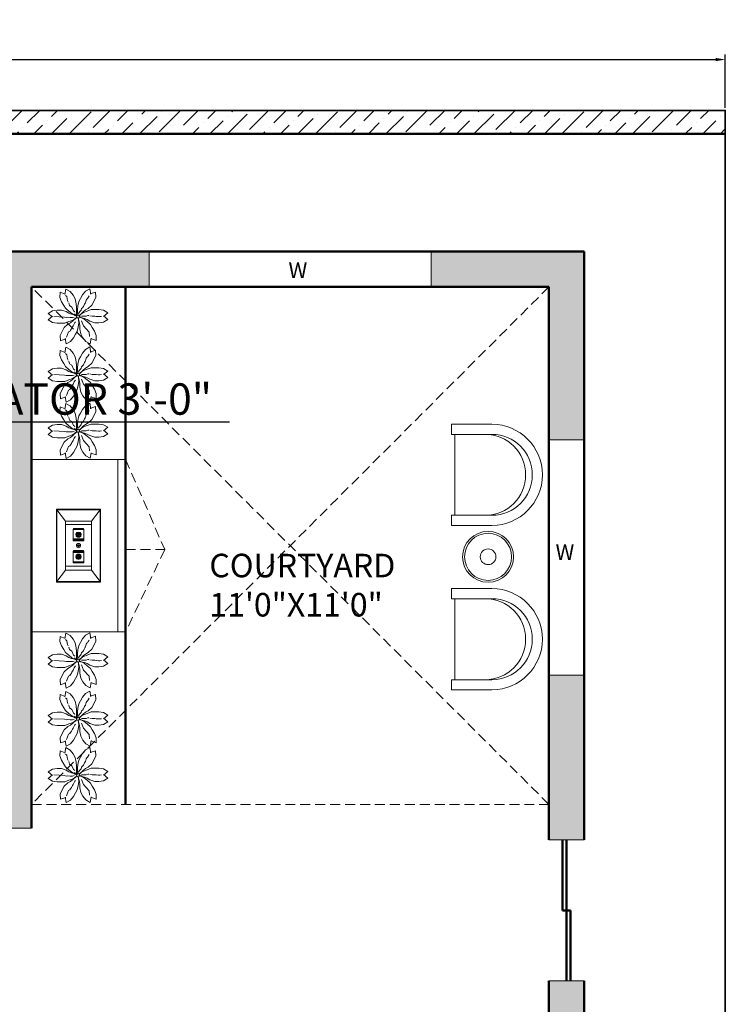
# Model space of a CAD drawing. Units: inches. Extents: x 3354 to 4308, y 1668 to 2317.
# Tile 8 of 11: x 3600 to 3780, y 2066 to 2317. Entities that reach past the tile are written whole.
import ezdxf

# ---------------------------------------------------------------- set-up
doc = ezdxf.new("R2010")
doc.units = ezdxf.units.IN
doc.linetypes.add('DASHED', pattern=[19.05, 12.7, -6.35])
for name, color, linetype, lineweight in [('A-ANNO-DIMS', 2, 'Continuous', 18), ('A-ANNO-TEXT', 7, 'Continuous', 18), ('A-AREA-IDEN', 3, 'Continuous', 18), ('A-FLOR-OVHD', 8, 'DASHED', 18), ('A-FURN', 8, 'Continuous', 18), ('A-GLAZ', 4, 'Continuous', 18), ('A-WALL', 7, 'Continuous', 50), ('A-WALL-PATT', 8, 'Continuous', 13), ('C-PROP', 1, 'Continuous', 35), ('L-PLNT', 84, 'Continuous', 13)]:
    doc.layers.add(name, color=color, linetype=linetype, lineweight=lineweight)
doc.styles.get("Standard").update_dxf_attribs({"font": 'arial.ttf'})
doc.dimstyles.new('ISO-25', dxfattribs={"dimtxt": 8, "dimasz": 2.5, "dimexe": 1.25, "dimexo": 0.625, "dimtad": 1, "dimdec": 1, "dimlunit": 3, "dimtxsty": 'Standard', "dimcen": 2.5, "dimadec": 0, "dimazin": 0, "dimtfac": 1, "dimtdec": 1, "dimtmove": 0, "dimatfit": 3, "dimfxl": 1, "dimarcsym": 0})

# ---------------------------------------------------------------- blocks, each defined once
blk = doc.blocks.new('12PSTG07')
at = {"color": 0, "linetype": 'ByBlock'}
for p, q in [((0, 15), (-12, 15)), ((0, 12), (0, 15)), ((-12, 12), (0, 12)), ((-1, -12), (-1, 12)), ((-12, -12), (0, -12)), ((0, -12), (0, -15)), ((0, -15), (-12, -15))]:
    blk.add_line(p, q, dxfattribs=at)
for centre, radius in [((-12, 0), 15), ((-12, 0), 12), ((-10, 0), 12)]:
    blk.add_arc(centre, radius, 90, 270, dxfattribs=at)
blk = doc.blocks.new('ml')
for p, q in [((3455.3311, 1925.7742), (3455.3307, 1925.7627)), ((3455.3431, 1925.7698), (3455.3311, 1925.7742)), ((3455.3419, 1925.7691), (3455.3441, 1925.7817)), ((3455.3435, 1925.7672), (3455.3464, 1925.7643)), ((3455.3441, 1925.7817), (3455.3543, 1925.7763)), ((3455.3543, 1925.7763), (3455.3608, 1925.7679)), ((3455.3608, 1925.7679), (3455.3657, 1925.7594)), ((3455.3826, 1925.7684), (3455.3777, 1925.76)), ((3455.3892, 1925.7768), (3455.3826, 1925.7684)), ((3455.3993, 1925.7823), (3455.3892, 1925.7768)), ((3455.3952, 1925.7623), (3455.3977, 1925.7658)), ((3455.4016, 1925.7697), (3455.3993, 1925.7823)), ((3455.4003, 1925.7704), (3455.4124, 1925.7747)), ((3455.4124, 1925.7747), (3455.4127, 1925.7632)), ((3455.3307, 1925.7627), (3455.3347, 1925.7528)), ((3455.3347, 1925.7528), (3455.3396, 1925.7443)), ((3455.3434, 1925.7376), (3455.3396, 1925.7443)), ((3455.3464, 1925.7643), (3455.3485, 1925.7554)), ((3455.3485, 1925.7554), (3455.3499, 1925.7524)), ((3455.3514, 1925.7499), (3455.3528, 1925.744)), ((3455.3528, 1925.744), (3455.3579, 1925.7405)), ((3455.3657, 1925.7594), (3455.368, 1925.7482)), ((3455.368, 1925.7482), (3455.3679, 1925.7458)), ((3455.3688, 1925.7419), (3455.3679, 1925.7458)), ((3455.3707, 1925.7348), (3455.3721, 1925.7432)), ((3455.3721, 1925.7432), (3455.3738, 1925.7534)), ((3455.3738, 1925.7534), (3455.3777, 1925.76)), ((3455.3848, 1925.7414), (3455.3855, 1925.743)), ((3455.3855, 1925.743), (3455.3866, 1925.7454)), ((3455.3866, 1925.7454), (3455.3873, 1925.7469)), ((3455.3873, 1925.7469), (3455.3888, 1925.7494)), ((3455.3888, 1925.7494), (3455.3895, 1925.7504)), ((3455.3895, 1925.7504), (3455.3912, 1925.7564)), ((3455.3912, 1925.7564), (3455.3927, 1925.7588)), ((3455.3927, 1925.7588), (3455.3938, 1925.7598)), ((3455.3938, 1925.7598), (3455.3952, 1925.7623)), ((3455.4038, 1925.7449), (3455.3952, 1925.7373)), ((3455.4087, 1925.7534), (3455.4038, 1925.7449)), ((3455.4127, 1925.7632), (3455.4087, 1925.7534)), ((3455.304, 1925.7261), (3455.3138, 1925.7322)), ((3455.3138, 1925.7178), (3455.304, 1925.7261)), ((3455.3138, 1925.7322), (3455.3243, 1925.7337)), ((3455.3243, 1925.7337), (3455.3341, 1925.7337)), ((3455.3341, 1925.7337), (3455.345, 1925.73)), ((3455.3514, 1925.7311), (3455.3434, 1925.7376)), ((3455.345, 1925.73), (3455.3509, 1925.7263)), ((3455.3509, 1925.7263), (3455.3573, 1925.7241)), ((3455.3579, 1925.7256), (3455.3514, 1925.7311)), ((3455.3573, 1925.7241), (3455.3659, 1925.7219)), ((3455.3579, 1925.7405), (3455.3622, 1925.7316)), ((3455.3656, 1925.7214), (3455.3579, 1925.7256)), ((3455.3622, 1925.7316), (3455.3639, 1925.7301)), ((3455.3639, 1925.7301), (3455.3647, 1925.7291)), ((3455.3643, 1925.7251), (3455.3672, 1925.7211)), ((3455.3707, 1925.7212), (3455.3656, 1925.7214)), ((3455.3659, 1925.7219), (3455.3697, 1925.7189)), ((3455.3688, 1925.7216), (3455.3688, 1925.7419)), ((3455.3691, 1925.7345), (3455.3715, 1925.726)), ((3455.3708, 1925.726), (3455.3707, 1925.7348)), ((3455.3715, 1925.726), (3455.3707, 1925.7212)), ((3455.3733, 1925.7215), (3455.3708, 1925.726)), ((3455.3778, 1925.7232), (3455.3733, 1925.7215)), ((3455.3736, 1925.7261), (3455.3765, 1925.7301)), ((3455.3748, 1925.7194), (3455.3775, 1925.7238)), ((3455.3765, 1925.7301), (3455.3776, 1925.7316)), ((3455.3775, 1925.7238), (3455.385, 1925.7283)), ((3455.3776, 1925.7316), (3455.3794, 1925.7335)), ((3455.384, 1925.7296), (3455.3778, 1925.7232)), ((3455.3794, 1925.7335), (3455.3805, 1925.737)), ((3455.3805, 1925.737), (3455.3826, 1925.739)), ((3455.3826, 1925.739), (3455.3848, 1925.7414)), ((3455.3891, 1925.734), (3455.384, 1925.7296)), ((3455.385, 1925.7283), (3455.393, 1925.7312)), ((3455.3952, 1925.7373), (3455.3891, 1925.734)), ((3455.3905, 1925.7196), (3455.3945, 1925.7211)), ((3455.393, 1925.7312), (3455.4026, 1925.7349)), ((3455.3945, 1925.7211), (3455.397, 1925.7211)), ((3455.3995, 1925.7206), (3455.4045, 1925.7196)), ((3455.4026, 1925.7349), (3455.4103, 1925.7348)), ((3455.4201, 1925.7348), (3455.4103, 1925.7348)), ((3455.4306, 1925.7333), (3455.4201, 1925.7348)), ((3455.4404, 1925.7273), (3455.4306, 1925.7333)), ((3455.4306, 1925.719), (3455.4404, 1925.7273)), ((3455.4306, 1925.7205), (3455.4404, 1925.7122)), ((3455.3138, 1925.7193), (3455.304, 1925.711)), ((3455.304, 1925.711), (3455.3138, 1925.705)), ((3455.3138, 1925.705), (3455.3243, 1925.7035)), ((3455.317, 1925.7192), (3455.341, 1925.7177)), ((3455.3243, 1925.7035), (3455.3341, 1925.7035)), ((3455.3418, 1925.7034), (3455.3341, 1925.7035)), ((3455.3406, 1925.6934), (3455.3492, 1925.701)), ((3455.341, 1925.7177), (3455.3453, 1925.7167)), ((3455.3514, 1925.7071), (3455.3418, 1925.7034)), ((3455.3453, 1925.7167), (3455.3489, 1925.7172)), ((3455.3489, 1925.7172), (3455.3543, 1925.7167)), ((3455.3492, 1925.701), (3455.3553, 1925.7043)), ((3455.3595, 1925.71), (3455.3514, 1925.7071)), ((3455.3543, 1925.7167), (3455.3597, 1925.7167)), ((3455.3553, 1925.7043), (3455.3605, 1925.7088)), ((3455.367, 1925.7145), (3455.3595, 1925.71)), ((3455.3597, 1925.7167), (3455.3636, 1925.7177)), ((3455.3605, 1925.7088), (3455.3667, 1925.7151)), ((3455.3608, 1925.6974), (3455.3618, 1925.6993)), ((3455.3618, 1925.6993), (3455.3632, 1925.7023)), ((3455.3632, 1925.7023), (3455.3647, 1925.7048)), ((3455.3647, 1925.7048), (3455.3661, 1925.7067)), ((3455.3667, 1925.7151), (3455.3712, 1925.7168)), ((3455.3697, 1925.7189), (3455.367, 1925.7145)), ((3455.3712, 1925.7168), (3455.3736, 1925.7123)), ((3455.3738, 1925.7035), (3455.3723, 1925.6951)), ((3455.373, 1925.7123), (3455.3737, 1925.7171)), ((3455.3753, 1925.7038), (3455.373, 1925.7123)), ((3455.3736, 1925.7123), (3455.3738, 1925.7035)), ((3455.3737, 1925.7171), (3455.3789, 1925.7169)), ((3455.3785, 1925.7164), (3455.3748, 1925.7194)), ((3455.3767, 1925.6971), (3455.3753, 1925.7038)), ((3455.3871, 1925.7142), (3455.3785, 1925.7164)), ((3455.3789, 1925.7169), (3455.3865, 1925.7127)), ((3455.3798, 1925.7196), (3455.383, 1925.7196)), ((3455.3804, 1925.7089), (3455.385, 1925.6972)), ((3455.383, 1925.7196), (3455.3905, 1925.7196)), ((3455.3865, 1925.7127), (3455.3931, 1925.7072)), ((3455.3935, 1925.712), (3455.3871, 1925.7142)), ((3455.3931, 1925.7072), (3455.4011, 1925.7007)), ((3455.3994, 1925.7083), (3455.3935, 1925.712)), ((3455.4103, 1925.7046), (3455.3994, 1925.7083)), ((3455.4011, 1925.7007), (3455.4048, 1925.694)), ((3455.4045, 1925.7196), (3455.4103, 1925.7196)), ((3455.4103, 1925.7196), (3455.4139, 1925.7192)), ((3455.4201, 1925.7046), (3455.4103, 1925.7046)), ((3455.4139, 1925.7192), (3455.4189, 1925.7187)), ((3455.4189, 1925.7187), (3455.4225, 1925.7187)), ((3455.4306, 1925.7061), (3455.4201, 1925.7046)), ((3455.4225, 1925.7187), (3455.426, 1925.7192)), ((3455.4404, 1925.7122), (3455.4306, 1925.7061)), ((3455.3317, 1925.6751), (3455.3357, 1925.6849)), ((3455.3357, 1925.6849), (3455.3406, 1925.6934)), ((3455.3457, 1925.6716), (3455.3504, 1925.6835)), ((3455.3504, 1925.6835), (3455.3532, 1925.6849)), ((3455.3532, 1925.6849), (3455.355, 1925.6874)), ((3455.355, 1925.6874), (3455.3575, 1925.6904)), ((3455.3575, 1925.6904), (3455.3582, 1925.6924)), ((3455.3582, 1925.6924), (3455.3597, 1925.6949)), ((3455.3597, 1925.6949), (3455.3608, 1925.6974)), ((3455.3618, 1925.6699), (3455.3667, 1925.6783)), ((3455.3706, 1925.6849), (3455.3667, 1925.6783)), ((3455.3723, 1925.6951), (3455.3706, 1925.6849)), ((3455.3764, 1925.6901), (3455.3767, 1925.6971)), ((3455.3787, 1925.6789), (3455.3764, 1925.6901)), ((3455.3836, 1925.6704), (3455.3787, 1925.6789)), ((3455.385, 1925.6972), (3455.3976, 1925.683)), ((3455.3976, 1925.683), (3455.3985, 1925.6734)), ((3455.4097, 1925.6855), (3455.4048, 1925.694)), ((3455.4137, 1925.6756), (3455.4097, 1925.6855)), ((3455.4134, 1925.6641), (3455.4137, 1925.6756)), ((3455.3321, 1925.6636), (3455.3317, 1925.6751)), ((3455.3441, 1925.6679), (3455.3321, 1925.6636)), ((3455.3429, 1925.6686), (3455.3451, 1925.656)), ((3455.3451, 1925.656), (3455.3553, 1925.6615)), ((3455.3553, 1925.6615), (3455.3618, 1925.6699)), ((3455.3902, 1925.662), (3455.3836, 1925.6704)), ((3455.4003, 1925.6566), (3455.3902, 1925.662)), ((3455.4026, 1925.6692), (3455.4003, 1925.6566)), ((3455.4013, 1925.6685), (3455.4134, 1925.6641))]:
    blk.add_line(p, q)
blk = doc.blocks.new('12PLMP48')
for p, q in [((-4.94, 8.22), (-5, 8.31)), ((-5, 8.31), (5, 8.31)), ((-5, -8.31), (-5, 8.31)), ((-2.96, 5.62), (-4.94, 8.22)), ((4.94, 8.22), (-4.94, 8.22)), ((-4.94, 8.22), (-4.94, -8.22)), ((2.96, 5.62), (4.94, 8.22)), ((5, 8.31), (4.94, 8.22)), ((4.94, 8.22), (4.94, -8.22)), ((5, 8.31), (5, -8.31)), ((-2.94, 5.59), (-3, 5.62)), ((-3, 5.62), (3, 5.62)), ((-3, -5.63), (-3, 5.62)), ((2.94, 5.59), (-2.94, 5.59)), ((-2.94, 5.59), (-2.94, -5.59)), ((2.94, 4.81), (-2.94, 4.81)), ((3, 5.62), (2.94, 5.59)), ((2.94, -5.59), (2.94, 5.59)), ((3, -5.63), (3, 5.62)), ((-1.13, 3.94), (-1.25, 3.81)), ((-1.13, 3.84), (-1.25, 3.72)), ((-1.25, 3.81), (-1.25, 1.22)), ((-1.25, 3.72), (1.25, 3.72)), ((1.13, 3.94), (-1.13, 3.94)), ((-1.13, 3.84), (-1.13, 3.94)), ((1.13, 3.84), (-1.13, 3.84)), ((-0.62, 2.61), (-0.4, 2.98)), ((0, 2.5), (-0.62, 2.61)), ((-0.54, 2.19), (-0.62, 2.61)), ((-0.38, 2.28), (-0.54, 2.19)), ((-0.32, 2.88), (-0.49, 2.59)), ((-0.49, 2.59), (-0.43, 2.25)), ((-0.43, 2.58), (-0.28, 2.83)), ((-0.38, 2.28), (-0.43, 2.58)), ((0, 3.12), (-0.4, 2.98)), ((-0.4, 2.98), (-0.32, 2.88)), ((0, 2.5), (-0.38, 2.28)), ((-0.15, 2.09), (-0.38, 2.28)), ((0, 3), (-0.32, 2.88)), ((-0.32, 2.88), (-0.32, 2.88)), ((-0.32, 2.88), (-0.28, 2.83)), ((-0.28, 2.83), (0, 2.94)), ((-0.28, 2.83), (0, 2.5)), ((-0.21, 1.91), (0, 2.5)), ((-0.08, 2.6), (-0.12, 2.52)), ((-0.12, 2.52), (-0.11, 2.44)), ((-0.11, 2.44), (-0.04, 2.38)), ((0, 2.62), (-0.08, 2.6)), ((-0.04, 2.38), (0.04, 2.38)), ((0, 2.5), (0, 3.12)), ((0, 3.12), (0.4, 2.98)), ((0.32, 2.88), (0, 3)), ((0, 2.94), (0.28, 2.83)), ((0, 2.5), (0.32, 2.88)), ((0.08, 2.6), (0, 2.62)), ((0.62, 2.61), (0, 2.5)), ((0.54, 2.19), (0, 2.5)), ((0, 2.5), (0.21, 1.91)), ((0.04, 2.38), (0.11, 2.44)), ((0.12, 2.52), (0.08, 2.6)), ((0.11, 2.44), (0.12, 2.52)), ((0.38, 2.28), (0.15, 2.09)), ((0.28, 2.83), (0.43, 2.58)), ((0.32, 2.88), (0.4, 2.98)), ((0.49, 2.59), (0.32, 2.88)), ((0.32, 2.88), (0.32, 2.88)), ((0.43, 2.58), (0.38, 2.28)), ((0.4, 2.98), (0.62, 2.61)), ((0.43, 2.25), (0.49, 2.59)), ((0.54, 2.19), (0.62, 2.61)), ((1.25, 3.81), (1.13, 3.94)), ((1.13, 3.84), (1.13, 3.94)), ((1.25, 3.72), (1.13, 3.84)), ((1.25, 1.22), (1.25, 3.81)), ((-1.13, 1.41), (-1.25, 1.53)), ((-1.25, 1.53), (1.25, 1.53)), ((-1.13, 1.25), (-1.25, 1.37)), ((-1.25, 1.22), (-1.13, 1.09)), ((1.13, 1.41), (-1.13, 1.41)), ((-1.13, 1.41), (-1.13, 1.09)), ((-1.13, 1.25), (1.13, 1.25)), ((-1.13, 1.09), (1.13, 1.09)), ((-0.54, 2.19), (-0.21, 1.91)), ((-0.49, -0.09), (-0.43, 0.25)), ((-0.43, 2.25), (-0.17, 2.03)), ((-0.43, 0.25), (-0.17, 0.47)), ((-0.22, 0.12), (-0.25, -0.04)), ((-0.09, 0.23), (-0.22, 0.12)), ((0.21, 1.91), (-0.21, 1.91)), ((-0.17, 2.03), (0.17, 2.03)), ((0.17, 0.47), (-0.17, 0.47)), ((0.15, 2.09), (-0.15, 2.09)), ((-0.12, -0.12), (-0.12, 0.12)), ((-0.12, 0.12), (0.12, 0.12)), ((-0.09, 0.23), (0.09, 0.23)), ((0.22, 0.12), (0.09, 0.23)), ((0.12, 0.12), (0.12, -0.12)), ((0.17, 2.03), (0.43, 2.25)), ((0.43, 0.25), (0.17, 0.47)), ((0.21, 1.91), (0.54, 2.19)), ((0.25, -0.04), (0.22, 0.12)), ((0.43, 0.25), (0.49, -0.09)), ((1.25, 1.53), (1.13, 1.41)), ((1.13, 1.09), (1.13, 1.41)), ((1.13, 1.25), (1.25, 1.37)), ((1.13, 1.09), (1.25, 1.22)), ((-1.25, -1.22), (-1.13, -1.09)), ((-1.25, -1.22), (-1.25, -3.81)), ((-1.13, -1.25), (-1.25, -1.38)), ((-1.13, -1.41), (-1.25, -1.53)), ((-1.25, -1.53), (1.25, -1.53)), ((-1.13, -1.41), (-1.13, -1.09)), ((-1.13, -1.09), (1.13, -1.09)), ((1.13, -1.25), (-1.13, -1.25)), ((1.13, -1.41), (-1.13, -1.41)), ((-0.54, -2.19), (-0.62, -2.61)), ((-0.21, -1.91), (-0.54, -2.19)), ((-0.54, -2.19), (0, -2.5)), ((-0.32, -0.38), (-0.49, -0.09)), ((-0.43, -2.25), (-0.17, -2.03)), ((-0.38, -2.28), (-0.15, -2.09)), ((-0.32, -0.38), (0, -0.5)), ((-0.16, -0.19), (-0.25, -0.04)), ((0.21, -1.91), (-0.21, -1.91)), ((0, -2.5), (-0.21, -1.91)), ((-0.17, -2.03), (0.17, -2.03)), ((0, -0.25), (-0.16, -0.19)), ((-0.15, -2.09), (0.15, -2.09)), ((0.12, -0.12), (-0.12, -0.12)), ((0.16, -0.19), (0, -0.25)), ((0.32, -0.38), (0, -0.5)), ((0, -2.5), (0.21, -1.91)), ((0.15, -2.09), (0.38, -2.28)), ((0.16, -0.19), (0.25, -0.04)), ((0.17, -2.03), (0.43, -2.25)), ((0.21, -1.91), (0.54, -2.19)), ((0.32, -0.38), (0.49, -0.09)), ((0.54, -2.19), (0.38, -2.28)), ((0.62, -2.61), (0.54, -2.19)), ((1.13, -1.41), (1.13, -1.09)), ((1.13, -1.09), (1.25, -1.22)), ((1.25, -1.38), (1.13, -1.25)), ((1.25, -1.53), (1.13, -1.41)), ((1.25, -3.81), (1.25, -1.22)), ((-1.13, -3.84), (-1.25, -3.72)), ((-1.25, -3.72), (1.25, -3.72)), ((-1.25, -3.81), (-1.13, -3.94)), ((-1.13, -3.94), (-1.13, -3.84)), ((1.13, -3.84), (-1.13, -3.84)), ((-1.13, -3.94), (1.13, -3.94)), ((0, -2.5), (-0.62, -2.61)), ((-0.62, -2.61), (-0.4, -2.98)), ((-0.49, -2.59), (-0.43, -2.25)), ((-0.32, -2.88), (-0.49, -2.59)), ((-0.43, -2.58), (-0.38, -2.28)), ((-0.28, -2.84), (-0.43, -2.58)), ((-0.4, -2.98), (-0.32, -2.88)), ((-0.4, -2.98), (0, -3.13)), ((-0.32, -2.88), (-0.28, -2.84)), ((0, -3), (-0.32, -2.88)), ((-0.28, -2.84), (-0.08, -2.6)), ((0, -2.94), (-0.28, -2.84)), ((-0.11, -2.44), (-0.12, -2.52)), ((-0.12, -2.52), (-0.08, -2.6)), ((-0.04, -2.38), (-0.11, -2.44)), ((-0.08, -2.6), (0, -2.5)), ((-0.08, -2.6), (0, -2.63)), ((0.04, -2.38), (-0.04, -2.38)), ((0.11, -2.44), (0, -2.5)), ((0, -3.13), (0, -2.5)), ((0, -2.5), (0.4, -2.98)), ((0.62, -2.61), (0, -2.5)), ((0, -2.63), (0.08, -2.6)), ((0.28, -2.84), (0, -2.94)), ((0.32, -2.88), (0, -3)), ((0, -3.13), (0.4, -2.98)), ((0.11, -2.44), (0.04, -2.38)), ((0.08, -2.6), (0.12, -2.52)), ((0.38, -2.28), (0.11, -2.44)), ((0.12, -2.52), (0.11, -2.44)), ((0.43, -2.58), (0.28, -2.84)), ((0.49, -2.59), (0.32, -2.88)), ((0.38, -2.28), (0.43, -2.58)), ((0.4, -2.98), (0.62, -2.61)), ((0.43, -2.25), (0.49, -2.59)), ((1.25, -3.72), (1.13, -3.84)), ((1.13, -3.94), (1.25, -3.81)), ((1.13, -3.94), (1.13, -3.84)), ((-4.94, -8.22), (-2.96, -5.63)), ((-2.94, -5.59), (-3, -5.63)), ((-3, -5.63), (3, -5.63)), ((2.94, -4.69), (-2.94, -4.69)), ((-2.94, -5.59), (2.94, -5.59)), ((3, -5.63), (2.94, -5.59)), ((2.96, -5.63), (4.94, -8.22)), ((-4.94, -8.22), (-5, -8.31)), ((5, -8.31), (-5, -8.31)), ((4.94, -8.22), (-4.94, -8.22)), ((4.94, -8.22), (5, -8.31))]:
    blk.add_line(p, q)
blk = doc.blocks.new('*D49')
at = {"layer": 'A-ANNO-DIMS', "color": 0, "lineweight": -2, "transparency": 16777216}
for p, q in [((3396.28, 2294.92), (3396.28, 2308.52)), ((3780.28, 2294.92), (3780.28, 2308.52)), ((3398.78, 2307.27), (3777.78, 2307.27))]:
    blk.add_line(p, q, dxfattribs=at)
at = {"layer": 'A-ANNO-DIMS', "color": 0, "transparency": 16777216}
for points in [[(3398.78, 2307.68), (3398.78, 2306.85), (3396.28, 2307.27)], [(3777.78, 2307.68), (3777.78, 2306.85), (3780.28, 2307.27)]]:
    blk.add_solid(points, dxfattribs=at)
at = {"layer": 'Defpoints', "color": 0, "transparency": 16777216}
for p in [(3780.28, 2307.27), (3396.28, 2294.3), (3780.28, 2294.3)]:
    blk.add_point(p, dxfattribs=at)
at = {"layer": 'A-ANNO-DIMS', "color": 0, "transparency": 16777216, "insert": (3588.28, 2311.98), "char_height": 8, "attachment_point": 5}
blk.add_mtext("32'", dxfattribs=at)
blk = doc.blocks.new('*D84')
at = {"layer": 'A-ANNO-DIMS', "color": 0, "lineweight": -2, "transparency": 16777216}
for p, q in [((3501.28, 2219.67), (3501.28, 2213.65)), ((3537.28, 2219.67), (3537.28, 2213.65)), ((3503.78, 2214.9), (3534.78, 2214.9)), ((3537.28, 2214.9), (3653.77, 2214.9))]:
    blk.add_line(p, q, dxfattribs=at)
at = {"layer": 'A-ANNO-DIMS', "color": 0, "transparency": 16777216}
for points in [[(3503.78, 2215.31), (3503.78, 2214.48), (3501.28, 2214.9)], [(3534.78, 2215.31), (3534.78, 2214.48), (3537.28, 2214.9)]]:
    blk.add_solid(points, dxfattribs=at)
at = {"layer": 'Defpoints', "color": 0, "transparency": 16777216}
for p in [(3501.28, 2220.3), (3537.28, 2220.3), (3537.28, 2214.9)]:
    blk.add_point(p, dxfattribs=at)
at = {"layer": 'A-ANNO-DIMS', "color": 0, "transparency": 16777216, "insert": (3596.78, 2219.66), "char_height": 8, "attachment_point": 5}
blk.add_mtext('REFRIGERATOR 3\'-0"', dxfattribs=at)

msp = doc.modelspace()

# ---------------------------------------------------------------- hatches: boundary and pattern name
at = {"layer": 'A-WALL-PATT', "transparency": 33554687}
h = msp.add_hatch(dxfattribs=at)
h.set_pattern_fill('ANSI36', color=256)
h.paths.add_polyline_path([(3780.28, 2294.3), (3396.28, 2294.3), (3396.28, 2258.3), (3405.28, 2258.3), (3405.28, 2288.3), (3780.28, 2288.3)])
h = msp.add_hatch(color=256, dxfattribs=at)
h.dxf.hatch_style = 1
h.paths.add_polyline_path([(3546.28, 1829.3), (3552.28, 1829.3), (3552.28, 1838.3), (3546.28, 1838.3), (3546.28, 1910.3), (3582.28, 1910.3), (3582.28, 1919.3), (3546.28, 1919.3), (3546.28, 1961.3), (3534.28, 1961.3), (3534.28, 1955.3), (3537.28, 1955.3), (3537.28, 1808.3), (3516.28, 1808.3), (3516.28, 1799.3), (3546.28, 1799.3)])
h.paths.add_polyline_path([(3672.28, 1919.3), (3656.51, 1919.3), (3630.28, 1919.3), (3630.28, 1910.3), (3642.28, 1910.3), (3642.28, 1838.3), (3630.28, 1838.3), (3630.28, 1835.3), (3630.28, 1829.3), (3642.28, 1829.3), (3642.28, 1799.3), (3651.28, 1799.3), (3651.28, 1910.3), (3672.28, 1910.3)])
h.paths.add_polyline_path([(3744.28, 1959.8), (3735.28, 1959.8), (3735.28, 1923.23), (3735.28, 1919.3), (3714.28, 1919.3), (3714.28, 1910.3), (3744.28, 1910.3)])
h.paths.add_polyline_path([(3744.28, 2072.3), (3735.28, 2072.3), (3735.28, 2031.8), (3744.28, 2031.8)])
h.paths.add_polyline_path([(3744.28, 2150.3), (3735.28, 2150.3), (3735.28, 2108.3), (3744.28, 2108.3)])
h.paths.add_polyline_path([(3744.28, 2258.3), (3705.28, 2258.3), (3705.28, 2249.3), (3735.28, 2249.3), (3735.28, 2210.3), (3744.28, 2210.3)])
h.paths.add_polyline_path([(3633.28, 2258.3), (3583.78, 2258.3), (3583.78, 2249.3), (3588.24, 2249.3), (3597.28, 2249.3), (3597.28, 2165.3), (3594.28, 2165.3), (3594.28, 2159.3), (3597.28, 2159.3), (3597.28, 2117.3), (3594.28, 2117.3), (3594.28, 2111.3), (3603.28, 2111.3), (3603.28, 2249.3), (3633.28, 2249.3)])
h.paths.add_polyline_path([(3559.78, 2258.3), (3492.28, 2258.3), (3492.28, 2249.3), (3537.28, 2249.3), (3537.28, 2117.3), (3534.28, 2117.3), (3534.28, 2111.3), (3564.28, 2111.3), (3564.28, 2117.3), (3546.28, 2117.3), (3546.28, 2159.3), (3564.28, 2159.3), (3564.28, 2165.3), (3546.28, 2165.3), (3546.28, 2249.3), (3559.78, 2249.3)])
h.paths.add_polyline_path([(3450.28, 2258.3), (3396.28, 2258.3), (3396.28, 1799.3), (3474.28, 1799.3), (3474.28, 1808.3), (3405.28, 1808.3), (3405.28, 1955.3), (3498.28, 1955.3), (3498.28, 1961.3), (3405.28, 1961.3), (3405.28, 2111.3), (3498.28, 2111.3), (3498.28, 2117.3), (3405.28, 2117.3), (3405.28, 2249.3), (3450.28, 2249.3)])
h.paths.add_polyline_path([(3582.28, 1838.3), (3576.28, 1838.3), (3576.28, 1829.3), (3582.28, 1829.3)], flags=17)

# ---------------------------------------------------------------- linework, layer by layer
at = {"layer": 'A-FLOR-OVHD', "ltscale": 0.2}
for p, q in [((3735.28, 2117.3), (3603.28, 2249.3)), ((3735.28, 2249.3), (3603.28, 2117.3)), ((3627.28, 2205.3), (3637.28, 2182.3)), ((3627.28, 2182.3), (3637.28, 2182.3)), ((3637.28, 2182.3), (3627.28, 2161.3)), ((3603.28, 2117.3), (3735.28, 2117.3))]:
    msp.add_line(p, q, dxfattribs=at)
at = {"layer": 'A-FURN'}
for p, q in [((3603.28, 2205.3), (3627.28, 2205.3)), ((3625.28, 2161.3), (3625.28, 2205.3)), ((3603.28, 2161.3), (3627.28, 2161.3))]:
    msp.add_line(p, q, dxfattribs=at)
for radius in [6.5, 6, 2]:
    msp.add_circle((3719.77, 2180.46), radius, dxfattribs=at)
at = {"layer": 'A-GLAZ'}
for p, q in [((3633.28, 2249.3), (3633.28, 2258.3)), ((3705.28, 2249.3), (3705.28, 2258.3)), ((3735.28, 2210.3), (3744.28, 2210.3)), ((3735.28, 2150.3), (3744.28, 2150.3)), ((3603.28, 2111.3), (3594.28, 2111.3)), ((3744.28, 2108.3), (3735.28, 2108.3)), ((3744.28, 2072.3), (3735.28, 2072.3))]:
    msp.add_line(p, q, dxfattribs=at)
at = {"layer": 'A-WALL'}
for p, q in [((3405.28, 2288.3), (3780.28, 2288.3)), ((3744.28, 2258.3), (3396.28, 2258.3)), ((3744.28, 2108.3), (3744.28, 2258.3)), ((3735.28, 2249.3), (3603.28, 2249.3)), ((3603.28, 2111.3), (3603.28, 2249.3)), ((3627.28, 2117.3), (3627.28, 2249.3)), ((3735.28, 2108.3), (3735.28, 2249.3)), ((3738.78, 2090.3), (3738.78, 2108.3)), ((3739.78, 2108.3), (3739.78, 2072.3)), ((3739.78, 2090.3), (3738.78, 2090.3)), ((3739.78, 2090.3), (3740.78, 2090.3)), ((3740.78, 2090.3), (3740.78, 2072.3)), ((3735.28, 1919.3), (3735.28, 2072.3)), ((3744.28, 1890.3), (3744.28, 2072.3))]:
    msp.add_line(p, q, dxfattribs=at)
at = {"layer": 'C-PROP'}
msp.add_lwpolyline([(3738.28, 1754.3), (3780.28, 1754.3), (3780.28, 2294.3), (3396.28, 2294.3), (3396.28, 1754.3), (3576.28, 1754.3)], dxfattribs=at)

# ---------------------------------------------------------------- block references
at = {"layer": 'A-FURN', "xscale": 0.8597921787217945, "yscale": 0.8597921787217945, "zscale": 0.8597921787217945, "rotation": 179.9999999999999}
for p in [(3710.41, 2201.37), (3710.41, 2159.45)]:
    msp.add_blockref('12PSTG07', p, dxfattribs=at)
at = {"layer": 'L-PLNT'}
for name, p, xscale, yscale, zscale in [('ml', (-381573.5, -212428.35), 111.4753012117704, 111.4753012117704, 111.4753012117704), ('ml', (-381573.5, -212443.19), 111.4753012117704, 111.4753012117704, 111.4753012117704), ('ml', (-381573.5, -212457.55), 111.4753012117704, 111.4753012117704, 111.4753012117704), ('12PLMP48', (3615.28, 2183.3), 1.115911277925004, 1.115911277925004, 1.115911277925004), ('ml', (-381573.5, -212516.1), 111.4753012117704, 111.4753012117704, 111.4753012117704), ('ml', (-381573.5, -212530.94), 111.4753012117704, 111.4753012117704, 111.4753012117704), ('ml', (-381573.5, -212545.3), 111.4753012117704, 111.4753012117704, 111.4753012117704)]:
    msp.add_blockref(name, p, dxfattribs=dict(at, xscale=xscale, yscale=yscale, zscale=zscale))

# ---------------------------------------------------------------- texts
at = {"layer": 'A-ANNO-TEXT', "char_height": 4, "attachment_point": 1}
for insert in [(3668.85, 2255.52), (3736.97, 2183.67)]:
    msp.add_mtext_dynamic_manual_height_columns('\\pxt6;{W}', width=32.7844, gutter_width=12.5, heights=[0], dxfattribs=dict(at, insert=insert))
at = {"layer": 'A-AREA-IDEN', "insert": (3648.65, 2181.24), "char_height": 6, "attachment_point": 1}
msp.add_mtext_dynamic_manual_height_columns('COURTYARD\\P11\'0"X11\'0"', width=74.5832, gutter_width=12.5, heights=[0], dxfattribs=at)

# ---------------------------------------------------------------- dimensions: what is measured, and where the dimension line sits
at = {"layer": 'A-ANNO-DIMS'}
dim = msp.add_linear_dim(base=(3780.28, 2307.27), p1=(3396.28, 2294.3), p2=(3780.28, 2294.3), dimstyle='ISO-25', override={"dimclrd": 0, "dimclre": 0, "dimclrt": 0}, dxfattribs=at)
dim.commit()
dim.dimension.update_dxf_attribs({"geometry": '*D49', "text_midpoint": (3588.28, 2311.98)})
dim = msp.add_linear_dim(base=(3537.28, 2214.9), p1=(3501.28, 2220.3), p2=(3537.28, 2220.3), text='REFRIGERATOR <>', dimstyle='ISO-25', override={"dimdec": 1, "dimrnd": 0, "dimzin": 1, "dimlunit": 4, "dimfrac": 2}, dxfattribs=at)
dim.commit()
dim.dimension.update_dxf_attribs({"geometry": '*D84', "text_midpoint": (3596.78, 2219.66)})

doc.saveas('drawing.dxf')
